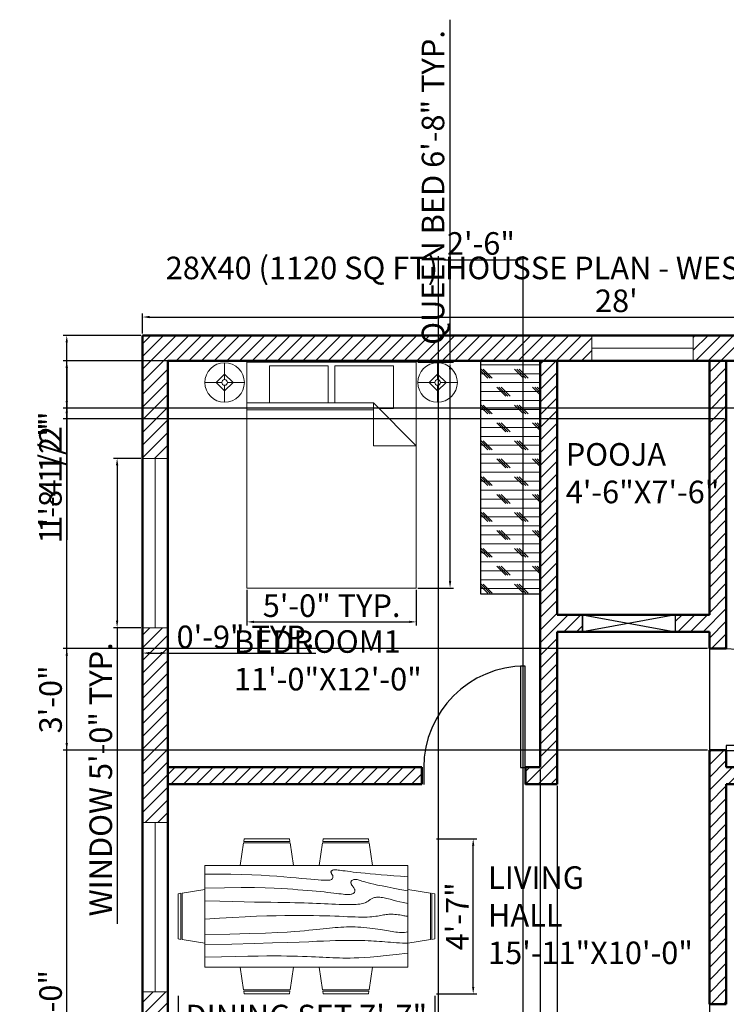
# Model space of a CAD drawing. Units: inches. Extents: x 1188 to 1681, y 1982 to 2608.
# Tile 3 of 4: x 1188 to 1439, y 2259 to 2608. Entities that reach past the tile are written whole.
import ezdxf

# ---------------------------------------------------------------- set-up
doc = ezdxf.new("R2010")
doc.units = ezdxf.units.IN
for name, color, linetype, lineweight in [('A-ANNO-DIMS', 2, 'Continuous', 18), ('A-ANNO-TEXT', 7, 'Continuous', 25), ('A-AREA-IDEN', 7, 'Continuous', 18), ('A-DOOR', 4, 'Continuous', 25), ('A-FLOR-CASE', 8, 'Continuous', 25), ('A-FLOR-CASE-PATT', 8, 'Continuous', 13), ('A-FURN', 8, 'Continuous', 18), ('A-GLAZ', 4, 'Continuous', 20), ('A-WALL', 7, 'Continuous', 50), ('A-WALL-PATT', 8, 'Continuous', 13)]:
    doc.layers.add(name, color=color, linetype=linetype, lineweight=lineweight)
doc.styles.get("Standard").update_dxf_attribs({"font": 'arial.ttf'})
doc.dimstyles.new('ISO-25', dxfattribs={"dimtxt": 8, "dimasz": 2.5, "dimexe": 1.25, "dimexo": 0.625, "dimtad": 1, "dimdec": 1, "dimlunit": 4, "dimtxsty": 'Standard', "dimcen": 2.5, "dimadec": 0, "dimazin": 0, "dimtfac": 1, "dimtdec": 1, "dimtmove": 0, "dimatfit": 3, "dimfxl": 1, "dimarcsym": 0})

# ---------------------------------------------------------------- blocks, each defined once
blk = doc.blocks.new('*U4')
for p, q in [((0, 0), (0, -6)), ((-36, 0), (-36, -6))]:
    blk.add_line(p, q)
blk.add_lwpolyline([(0, 0), (0, 36), (-1.75, 36), (-1.75, 0)], close=True)
blk.add_arc((0, 0), 36, 90, 180)
blk = doc.blocks.new('*U5')
for p, q in [((0, 0), (0, 6)), ((36, 0), (36, 6))]:
    blk.add_line(p, q)
blk.add_lwpolyline([(0, 0), (0, -36), (1.75, -36), (1.75, 0)], close=True)
blk.add_arc((0, 0), 36, 270, 0)
blk = doc.blocks.new('Bed - Queen')
for p, q in [((0, -80.00003), (0, 0)), ((0, 0), (59.99999, 0)), ((59.99999, 0), (59.99999, -80.00003)), ((7.99999, -1.2), (28.79998, -1.2)), ((7.99999, -14.4), (7.99999, -1.2)), ((28.79998, -1.2), (28.79998, -14.4)), ((31.19999, -1.2), (51.99999, -1.2)), ((31.19999, -14.4), (31.19999, -1.2)), ((51.99999, -1.2), (51.99999, -16.4)), ((0, -14.4), (44.8, -14.4)), ((44.8, -16.8), (0, -16.8)), ((59.99999, -29.6), (44.8, -14.4)), ((44.8, -14.4), (44.8, -29.6)), ((51.99999, -16.4), (46.79936, -16.4)), ((44.8, -29.6), (59.99999, -29.6)), ((59.99999, -80.00003), (0, -80.00003))]:
    blk.add_line(p, q)
blk = doc.blocks.new('Dining Set - 36 x 72 in.')
for p, q in [((-22.2343, 26.00059), (-23.4847, 17.99762)), ((-22.2304, 26), (-5.7608, 26)), ((-22, 27.5), (-22.1562, 26.50042)), ((-5.8416, 26.5), (-22.1534, 26.5)), ((-22, 27.5), (-6, 27.5)), ((-5.8437, 26.49966), (-6, 27.5)), ((-4.5152, 17.99762), (-5.7655, 25.99926)), ((5.7657, 26.00059), (4.5153, 17.99762)), ((5.7696, 26), (22.2392, 26)), ((6, 27.5), (5.8438, 26.50042)), ((22.1584, 26.5), (5.8466, 26.5)), ((6, 27.5), (22, 27.5)), ((22.1563, 26.49966), (22, 27.5)), ((23.4848, 17.99762), (22.2345, 25.99926)), ((36, 18), (-36, 18)), ((-36, 18), (-36, -18)), ((36, -18), (36, 18)), ((-45.5, 8), (-44.5004, 8.15617)), ((-45.5, 8), (-45.5, -8)), ((-44.5, -8.15843), (-44.5, 8.15338)), ((-44.0006, 8.23428), (-35.9976, 9.48474)), ((-44, 8.23041), (-44, -8.23915)), ((44.0006, 8.23428), (35.9976, 9.48474)), ((44, 8.23041), (44, -8.23915)), ((44.5, -8.15843), (44.5, 8.15338)), ((45.5, 8), (44.5005, 8.15617)), ((45.5, 8), (45.5, -8)), ((-44.4997, -8.15631), (-45.5, -8)), ((-35.9976, -9.48476), (-43.9993, -8.2345)), ((35.9976, -9.48476), (43.9993, -8.2345)), ((44.4997, -8.15631), (45.5, -8)), ((-36, -18), (36, -18)), ((-22.2343, -26.0006), (-23.4847, -17.99762)), ((-4.5152, -17.99762), (-5.7655, -25.99928)), ((5.7657, -26.0006), (4.5153, -17.99762)), ((23.4848, -17.99762), (22.2345, -25.99928)), ((-22.2304, -26), (-5.7608, -26)), ((-22, -27.5), (-22.1562, -26.50044)), ((-5.8416, -26.5), (-22.1534, -26.5)), ((-22, -27.5), (-6, -27.5)), ((-5.8437, -26.49967), (-6, -27.5)), ((5.7696, -26), (22.2392, -26)), ((6, -27.5), (5.8438, -26.50044)), ((22.1584, -26.5), (5.8466, -26.5)), ((6, -27.5), (22, -27.5)), ((22.1563, -26.49967), (22, -27.5))]:
    blk.add_line(p, q)
for points in [[(-36, 15), (-31.1772, 14.97754), (-26.8079, 14.91406), (-22.8538, 14.81543), (-19.276, 14.6875), (-16.0362, 14.53613), (-13.0957, 14.36718), (-10.4159, 14.18652), (-7.9583, 14), (-5.6904, 13.81315), (-3.6035, 13.63021), (-1.6954, 13.45508), (0.0365, 13.29166), (1.5945, 13.14388), (2.9811, 13.01562), (4.1988, 12.9108), (5.25, 12.83333), (6.1393, 12.78613), (6.8802, 12.76823), (7.4883, 12.77767), (7.9792, 12.8125), (8.3685, 12.87077), (8.6719, 12.95052), (8.9049, 13.0498), (9.0833, 13.16666), (9.2205, 13.29899), (9.3216, 13.44401), (9.3895, 13.59879), (9.4271, 13.76041), (9.4373, 13.92594), (9.4232, 14.09245), (9.3875, 14.257), (9.3333, 14.41666), (9.2638, 14.56917), (9.1836, 14.71484), (9.0975, 14.85465), (9.0104, 14.98958), (8.9272, 15.1206), (8.8529, 15.2487), (8.7922, 15.37483), (8.75, 15.5), (8.7305, 15.62467), (8.7344, 15.74739), (8.7617, 15.86621), (8.8125, 15.97916), (8.8867, 16.08431), (8.9844, 16.17968), (9.1055, 16.26334), (9.25, 16.33333), (9.4189, 16.38802), (9.6172, 16.42708), (9.8506, 16.45052), (10.125, 16.45833), (10.4463, 16.45052), (10.8203, 16.42708), (11.2529, 16.38802), (11.75, 16.33333), (12.3184, 16.26318), (12.9694, 16.17838), (13.7151, 16.07991), (14.5677, 15.96875), (15.5395, 15.84586), (16.6426, 15.71224), (17.8893, 15.56884), (19.2917, 15.41666), (20.859, 15.25667), (22.5879, 15.08984), (24.4721, 14.91715), (26.5052, 14.73958), (28.6809, 14.5581), (30.9929, 14.3737), (33.4347, 14.18733), (36, 14)], [(-36, 10), (-28.9766, 10.14274), (-23.1725, 10.20442), (-18.4241, 10.19775), (-14.5677, 10.13541), (-11.4399, 10.03011), (-8.877, 9.89453), (-6.7154, 9.74137), (-4.7917, 9.58333), (-2.9698, 9.43082), (-1.2246, 9.28515), (0.4415, 9.14534), (2.026, 9.01041), (3.5266, 8.87939), (4.9408, 8.7513), (6.266, 8.62516), (7.5, 8.5), (8.6411, 8.37549), (9.6914, 8.2539), (10.6538, 8.13818), (11.5312, 8.03125), (12.3267, 7.93603), (13.043, 7.85547), (13.6831, 7.79248), (14.25, 7.75), (14.7471, 7.7303), (15.1797, 7.73307), (15.5537, 7.75732), (15.875, 7.80208), (16.1494, 7.86637), (16.3828, 7.94922), (16.5811, 8.04964), (16.75, 8.16666), (16.8944, 8.29915), (17.0143, 8.44531), (17.1089, 8.60319), (17.1771, 8.77083), (17.218, 8.94629), (17.2305, 9.1276), (17.2137, 9.31282), (17.1667, 9.5), (17.0895, 9.6875), (16.987, 9.875), (16.8649, 10.0625), (16.7292, 10.25), (16.5856, 10.4375), (16.4401, 10.625), (16.2985, 10.8125), (16.1667, 11), (16.05, 11.18733), (15.9518, 11.3737), (15.8752, 11.5581), (15.8229, 11.73958), (15.798, 11.91715), (15.8034, 12.08984), (15.842, 12.25667), (15.9167, 12.41666), (16.0295, 12.56836), (16.1784, 12.70833), (16.3605, 12.83268), (16.5729, 12.9375), (16.8127, 13.01888), (17.0768, 13.07291), (17.3625, 13.0957), (17.6667, 13.08333), (17.9894, 13.03312), (18.3418, 12.94726), (18.7382, 12.82918), (19.1927, 12.68229), (19.7195, 12.51001), (20.3327, 12.31575), (21.0465, 12.10294), (21.875, 11.875), (22.8357, 11.63354), (23.959, 11.37304), (25.2786, 11.08618), (26.8282, 10.76562), (28.6414, 10.40405), (30.752, 9.99414), (33.1936, 9.52856), (36, 9)], [(-36, 5.5), (-30.7157, 5.3348), (-26.069, 5.20963), (-21.9946, 5.11767), (-18.4271, 5.05208), (-15.3009, 5.00602), (-12.5508, 4.97265), (-10.1112, 4.94515), (-7.9167, 4.91666), (-5.909, 4.88167), (-4.0586, 4.83984), (-2.3429, 4.79215), (-0.7396, 4.73958), (0.7739, 4.6831), (2.22, 4.6237), (3.6213, 4.56233), (5, 4.5), (6.373, 4.43782), (7.7344, 4.3776), (9.0723, 4.32129), (10.375, 4.27083), (11.6309, 4.22819), (12.8281, 4.19531), (13.9551, 4.17415), (15, 4.16666), (15.954, 4.17448), (16.819, 4.19791), (17.6001, 4.23698), (18.3021, 4.29166), (18.9299, 4.36198), (19.4883, 4.44791), (19.9823, 4.54948), (20.4167, 4.66666), (20.7969, 4.79899), (21.1302, 4.94401), (21.4245, 5.09879), (21.6875, 5.26041), (21.9271, 5.42594), (22.1511, 5.59245), (22.3672, 5.757), (22.5834, 5.91666), (22.8065, 6.06868), (23.0404, 6.21093), (23.2879, 6.34147), (23.5521, 6.45833), (23.8358, 6.55957), (24.142, 6.64323), (24.4735, 6.70735), (24.8334, 6.75), (25.2235, 6.76969), (25.642, 6.76692), (26.0858, 6.74267), (26.5521, 6.69791), (27.0379, 6.63362), (27.5404, 6.55078), (28.0565, 6.45036), (28.5834, 6.33333), (29.1242, 6.19987), (29.7071, 6.04687), (30.3661, 5.87044), (31.1354, 5.66666), (32.0493, 5.43164), (33.142, 5.16146), (34.4475, 4.85221), (36, 4.5)], [(-36, -1), (-30.7915, -0.6591), (-26.0195, -0.38216), (-21.6519, -0.16284), (-17.6563, 0.00521), (-14.0005, 0.12833), (-10.6523, 0.21289), (-7.5796, 0.26522), (-4.75, 0.29166), (-2.134, 0.29793), (0.2878, 0.28711), (2.5317, 0.26163), (4.6146, 0.22396), (6.5529, 0.17651), (8.3633, 0.12174), (10.0623, 0.06209), (11.6667, 0), (13.1899, -0.06201), (14.6341, -0.1211), (15.9982, -0.17432), (17.2813, -0.21875), (18.4823, -0.25147), (19.6003, -0.26953), (20.6343, -0.27002), (21.5834, -0.25), (22.4481, -0.20768), (23.2357, -0.14584), (23.9549, -0.06836), (24.6146, 0.02083), (25.2235, 0.11784), (25.7904, 0.21875), (26.3241, 0.31966), (26.8334, 0.41666), (27.3265, 0.50618), (27.8099, 0.58593), (28.2894, 0.65397), (28.7709, 0.70833), (29.2601, 0.74707), (29.763, 0.76823), (30.2855, 0.76985), (30.8334, 0.75), (31.4088, 0.70784), (31.9994, 0.64713), (32.589, 0.57275), (33.1615, 0.48958), (33.7008, 0.4025), (34.1908, 0.3164), (34.6153, 0.23616), (34.9584, 0.16666), (35.2099, 0.11165), (35.3848, 0.07031), (35.504, 0.04069), (35.5886, 0.02083), (35.6594, 0.00879), (35.7377, 0.0026), (35.8442, 0.00032), (36, 0)], [(-36, -6.5), (-27.1843, -6.31267), (-20.084, -6.1263), (-14.469, -5.9419), (-10.1094, -5.76042), (-6.7752, -5.58285), (-4.2363, -5.41016), (-2.2629, -5.24333), (-0.625, -5.08334), (0.8708, -4.93099), (2.2715, -4.78646), (3.5872, -4.64974), (4.8281, -4.52084), (6.0046, -4.39974), (7.127, -4.28646), (8.2053, -4.18099), (9.25, -4.08334), (10.2705, -3.99382), (11.2734, -3.91407), (12.2647, -3.84603), (13.25, -3.79167), (14.2354, -3.75293), (15.2266, -3.73177), (16.2295, -3.73015), (17.25, -3.75), (18.2912, -3.79248), (19.3451, -3.85547), (20.4009, -3.93604), (21.4479, -4.03125), (22.4754, -4.13819), (23.4727, -4.25391), (24.4289, -4.37549), (25.3334, -4.5), (26.1785, -4.62492), (26.9694, -4.74935), (27.7145, -4.87281), (28.4219, -4.99479), (29.1, -5.11483), (29.7572, -5.23242), (30.4016, -5.34709), (31.0417, -5.45834), (31.6837, -5.56437), (32.3262, -5.65821), (32.9658, -5.73153), (33.599, -5.77604), (34.2224, -5.78345), (34.8327, -5.74545), (35.4264, -5.65373), (36, -5.5)], [(-36, -10), (-26.4022, -9.81299), (-18.4675, -9.62891), (-11.9839, -9.45069), (-6.7396, -9.28125), (-2.5226, -9.12354), (0.8789, -8.98047), (3.6769, -8.85498), (6.0833, -8.75), (8.2767, -8.66765), (10.3021, -8.60677), (12.1712, -8.56543), (13.8958, -8.54167), (15.4876, -8.53353), (16.9583, -8.53907), (18.3197, -8.55632), (19.5834, -8.58334), (20.7616, -8.61841), (21.8685, -8.66081), (22.9188, -8.71004), (23.9271, -8.76563), (24.9081, -8.82707), (25.8763, -8.89388), (26.8465, -8.96558), (27.8334, -9.04167), (28.8474, -9.12118), (29.8828, -9.20117), (30.93, -9.27824), (31.9792, -9.34896), (33.0205, -9.40991), (34.0443, -9.45768), (35.0407, -9.48885), (36, -9.5)], [(-36, -14.5), (-30.0881, -14.33513), (-25.0332, -14.21224), (-20.7312, -14.12647), (-17.0781, -14.07292), (-13.97, -14.04671), (-11.3027, -14.04297), (-8.9724, -14.05681), (-6.875, -14.08334), (-4.9224, -14.11833), (-3.0905, -14.16016), (-1.3709, -14.20785), (0.2448, -14.26042), (1.7647, -14.3169), (3.1973, -14.3763), (4.5507, -14.43767), (5.8333, -14.5), (7.0554, -14.5621), (8.235, -14.62175), (9.3922, -14.67652), (10.5469, -14.72396), (11.7192, -14.76164), (12.929, -14.78711), (14.1965, -14.79794), (15.5417, -14.79167), (16.9933, -14.76424), (18.6152, -14.70508), (20.4804, -14.60197), (22.6615, -14.44271), (25.2312, -14.21509), (28.2624, -13.9069), (31.8277, -13.50594), (36, -13)]]:
    blk.add_lwpolyline(points)
blk = doc.blocks.new('Lamp - Table')
for p, q in [((0, 7), (0, 1)), ((-1, 0), (-7, 0)), ((0, 3), (-3, 0)), ((-3, 0), (0, -3)), ((3, 0), (0, 3)), ((0, -3), (3, 0)), ((1, 0), (7, 0)), ((0, -1), (0, -7))]:
    blk.add_line(p, q)
for radius in [7, 1]:
    blk.add_circle((0, 0), radius)
blk = doc.blocks.new('*D14')
at = {"layer": 'A-ANNO-DIMS', "color": 0, "lineweight": -2, "transparency": 16777216}
for p, q in [((1231.72, 2497.04), (1231.72, 2504.18)), ((1234.22, 2502.93), (1565.22, 2502.93)), ((1567.72, 2497.04), (1567.72, 2504.18))]:
    blk.add_line(p, q, dxfattribs=at)
at = {"layer": 'A-ANNO-DIMS', "color": 0, "transparency": 16777216}
for points in [[(1234.22, 2503.35), (1234.22, 2502.52), (1231.72, 2502.93)], [(1565.22, 2503.35), (1565.22, 2502.52), (1567.72, 2502.93)]]:
    blk.add_solid(points, dxfattribs=at)
at = {"layer": 'Defpoints', "color": 0, "transparency": 16777216}
for p in [(1567.72, 2502.93), (1231.72, 2496.41), (1567.72, 2496.41)]:
    blk.add_point(p, dxfattribs=at)
at = {"layer": 'A-ANNO-DIMS', "color": 0, "transparency": 16777216, "insert": (1399.72, 2507.64), "char_height": 8, "attachment_point": 5}
blk.add_mtext("28'", dxfattribs=at)
blk = doc.blocks.new('WIN-60IN')
for p, q in [((0, 9), (0, 0)), ((60, 0), (60, 9)), ((60, 9), (60, 4.5)), ((60, 4.5), (0, 4.5)), ((0, 0), (60, 0))]:
    blk.add_line(p, q)
blk = doc.blocks.new('*D24')
at = {"layer": 'A-ANNO-DIMS', "color": 0, "lineweight": -2, "transparency": 16777216}
for p, q in [((1231.09, 2452.82), (1221.47, 2452.82)), ((1222.72, 2450.32), (1222.72, 2395.32)), ((1231.09, 2392.82), (1221.47, 2392.82)), ((1222.72, 2392.82), (1222.72, 2287.84))]:
    blk.add_line(p, q, dxfattribs=at)
at = {"layer": 'A-ANNO-DIMS', "color": 0, "transparency": 16777216}
for points in [[(1222.3, 2450.32), (1223.13, 2450.32), (1222.72, 2452.82)], [(1222.3, 2395.32), (1223.13, 2395.32), (1222.72, 2392.82)]]:
    blk.add_solid(points, dxfattribs=at)
at = {"layer": 'Defpoints', "color": 0, "transparency": 16777216}
for p in [(1231.72, 2452.82), (1222.72, 2392.82), (1231.72, 2392.82)]:
    blk.add_point(p, dxfattribs=at)
at = {"layer": 'A-ANNO-DIMS', "color": 0, "transparency": 16777216, "insert": (1217.95, 2339.08), "char_height": 8, "attachment_point": 5, "rotation": 90}
blk.add_mtext('WINDOW 5\'-0" TYP.', dxfattribs=at)
blk = doc.blocks.new('*D25')
at = {"layer": 'A-ANNO-DIMS', "color": 0, "lineweight": -2, "transparency": 16777216}
for p, q in [((1231.72, 2392.2), (1231.72, 2382.57)), ((1240.72, 2392.2), (1240.72, 2382.57)), ((1234.22, 2383.82), (1238.22, 2383.82)), ((1240.72, 2383.82), (1293.23, 2383.82))]:
    blk.add_line(p, q, dxfattribs=at)
at = {"layer": 'A-ANNO-DIMS', "color": 0, "transparency": 16777216}
for points in [[(1234.22, 2384.24), (1234.22, 2383.41), (1231.72, 2383.82)], [(1238.22, 2384.24), (1238.22, 2383.41), (1240.72, 2383.82)]]:
    blk.add_solid(points, dxfattribs=at)
at = {"layer": 'Defpoints', "color": 0, "transparency": 16777216}
for p in [(1231.72, 2392.82), (1240.72, 2392.82), (1240.72, 2383.82)]:
    blk.add_point(p, dxfattribs=at)
at = {"layer": 'A-ANNO-DIMS', "color": 0, "transparency": 16777216, "insert": (1268.22, 2388.53), "char_height": 8, "attachment_point": 5}
blk.add_mtext('0\'-9" TYP.', dxfattribs=at)
blk = doc.blocks.new('*D28')
at = {"layer": 'A-ANNO-DIMS', "color": 0, "lineweight": -2, "transparency": 16777216}
for p, q in [((1340.77, 2486.88), (1340.77, 2608.31)), ((1329.39, 2486.88), (1342.02, 2486.88)), ((1340.77, 2409.38), (1340.77, 2484.38)), ((1329.39, 2406.88), (1342.02, 2406.88))]:
    blk.add_line(p, q, dxfattribs=at)
at = {"layer": 'A-ANNO-DIMS', "color": 0, "transparency": 16777216}
for points in [[(1340.35, 2484.38), (1341.18, 2484.38), (1340.77, 2486.88)], [(1340.35, 2409.38), (1341.18, 2409.38), (1340.77, 2406.88)]]:
    blk.add_solid(points, dxfattribs=at)
at = {"layer": 'Defpoints', "color": 0, "transparency": 16777216}
for p in [(1328.77, 2486.88), (1340.77, 2486.88), (1328.77, 2406.88)]:
    blk.add_point(p, dxfattribs=at)
at = {"layer": 'A-ANNO-DIMS', "color": 0, "transparency": 16777216, "insert": (1335.76, 2548.85), "char_height": 8, "attachment_point": 5, "rotation": 90}
blk.add_mtext('QUEEN BED 6\'-8" TYP.', dxfattribs=at)
blk = doc.blocks.new('*D29')
at = {"layer": 'A-ANNO-DIMS', "color": 0, "lineweight": -2, "transparency": 16777216}
for p, q in [((1268.77, 2406.26), (1268.77, 2393.63)), ((1328.77, 2406.26), (1328.77, 2393.63)), ((1271.27, 2394.88), (1326.27, 2394.88))]:
    blk.add_line(p, q, dxfattribs=at)
at = {"layer": 'A-ANNO-DIMS', "color": 0, "transparency": 16777216}
for points in [[(1271.27, 2395.3), (1271.27, 2394.47), (1268.77, 2394.88)], [(1326.27, 2395.3), (1326.27, 2394.47), (1328.77, 2394.88)]]:
    blk.add_solid(points, dxfattribs=at)
at = {"layer": 'Defpoints', "color": 0, "transparency": 16777216}
for p in [(1268.77, 2406.88), (1328.77, 2406.88), (1328.77, 2394.88)]:
    blk.add_point(p, dxfattribs=at)
at = {"layer": 'A-ANNO-DIMS', "color": 0, "transparency": 16777216, "insert": (1298.77, 2399.59), "char_height": 8, "attachment_point": 5}
blk.add_mtext('5\'-0" TYP.', dxfattribs=at)
blk = doc.blocks.new('*D38')
at = {"layer": 'A-ANNO-DIMS', "color": 0, "lineweight": -2, "transparency": 16777216}
for p, q in [((1244.32, 2262.4), (1244.32, 2248.12)), ((1335.32, 2262.4), (1335.32, 2248.12)), ((1246.82, 2249.37), (1332.82, 2249.37))]:
    blk.add_line(p, q, dxfattribs=at)
at = {"layer": 'A-ANNO-DIMS', "color": 0, "transparency": 16777216}
for points in [[(1246.82, 2249.79), (1246.82, 2248.96), (1244.32, 2249.37)], [(1332.82, 2249.79), (1332.82, 2248.96), (1335.32, 2249.37)]]:
    blk.add_solid(points, dxfattribs=at)
at = {"layer": 'Defpoints', "color": 0, "transparency": 16777216}
for p in [(1244.32, 2263.02), (1335.32, 2263.02), (1335.32, 2249.37)]:
    blk.add_point(p, dxfattribs=at)
at = {"layer": 'A-ANNO-DIMS', "color": 0, "transparency": 16777216, "insert": (1289.82, 2254.14), "char_height": 8, "attachment_point": 5}
blk.add_mtext('DINING SET 7\'-7"', dxfattribs=at)
blk = doc.blocks.new('*D39')
at = {"layer": 'A-ANNO-DIMS', "color": 0, "lineweight": -2, "transparency": 16777216}
for p, q in [((1335.95, 2318.02), (1350.22, 2318.02)), ((1348.97, 2265.52), (1348.97, 2315.52)), ((1335.95, 2263.02), (1350.22, 2263.02))]:
    blk.add_line(p, q, dxfattribs=at)
at = {"layer": 'A-ANNO-DIMS', "color": 0, "transparency": 16777216}
for points in [[(1348.56, 2315.52), (1349.39, 2315.52), (1348.97, 2318.02)], [(1348.56, 2265.52), (1349.39, 2265.52), (1348.97, 2263.02)]]:
    blk.add_solid(points, dxfattribs=at)
at = {"layer": 'Defpoints', "color": 0, "transparency": 16777216}
for p in [(1335.32, 2318.02), (1348.97, 2318.02), (1335.32, 2263.02)]:
    blk.add_point(p, dxfattribs=at)
at = {"layer": 'A-ANNO-DIMS', "color": 0, "transparency": 16777216, "insert": (1344.35, 2290.52), "char_height": 8, "attachment_point": 5, "rotation": 90}
blk.add_mtext('4\'-7"', dxfattribs=at)
blk = doc.blocks.new('*D44')
at = {"layer": 'A-ANNO-DIMS', "color": 0, "lineweight": -2, "transparency": 16777216}
for p, q in [((1231.09, 2496.41), (1203.62, 2496.41)), ((1204.87, 2018.91), (1204.87, 2493.91)), ((1231.09, 2016.41), (1203.62, 2016.41))]:
    blk.add_line(p, q, dxfattribs=at)
at = {"layer": 'A-ANNO-DIMS', "color": 0, "transparency": 16777216}
for points in [[(1204.45, 2493.91), (1205.28, 2493.91), (1204.87, 2496.41)], [(1204.45, 2018.91), (1205.28, 2018.91), (1204.87, 2016.41)]]:
    blk.add_solid(points, dxfattribs=at)
at = {"layer": 'Defpoints', "color": 0, "transparency": 16777216}
for p in [(1204.87, 2496.41), (1231.72, 2496.41), (1231.72, 2016.41)]:
    blk.add_point(p, dxfattribs=at)
at = {"layer": 'A-ANNO-DIMS', "color": 0, "transparency": 16777216, "insert": (1200.16, 2256.41), "char_height": 8, "attachment_point": 5, "rotation": 90}
blk.add_mtext('40\'-0"', dxfattribs=at)
blk = doc.blocks.new('*D47')
at = {"layer": 'A-ANNO-DIMS', "color": 0, "lineweight": -2, "transparency": 16777216}
for p, q in [((1336.72, 2164.04), (1336.72, 2524.51)), ((1339.22, 2523.26), (1364.22, 2523.26)), ((1366.72, 2164.04), (1366.72, 2524.51))]:
    blk.add_line(p, q, dxfattribs=at)
at = {"layer": 'A-ANNO-DIMS', "color": 0, "transparency": 16777216}
for points in [[(1339.22, 2523.68), (1339.22, 2522.85), (1336.72, 2523.26)], [(1364.22, 2523.68), (1364.22, 2522.85), (1366.72, 2523.26)]]:
    blk.add_solid(points, dxfattribs=at)
at = {"layer": 'Defpoints', "color": 0, "transparency": 16777216}
for p in [(1366.72, 2523.26), (1336.72, 2163.41), (1366.72, 2163.41)]:
    blk.add_point(p, dxfattribs=at)
at = {"layer": 'A-ANNO-DIMS', "color": 0, "transparency": 16777216, "insert": (1351.72, 2527.97), "char_height": 8, "attachment_point": 5}
blk.add_mtext('2\'-6"', dxfattribs=at)
blk = doc.blocks.new('*D50')
at = {"layer": 'A-ANNO-DIMS', "color": 0, "lineweight": -2, "transparency": 16777216}
for p, q in [((1372.72, 2342.79), (1372.72, 1988.31)), ((1378.72, 2336.79), (1378.72, 1988.31)), ((1370.22, 1989.56), (1367.72, 1989.56)), ((1372.72, 1989.56), (1378.72, 1989.56)), ((1381.22, 1989.56), (1406.23, 1989.56))]:
    blk.add_line(p, q, dxfattribs=at)
at = {"layer": 'A-ANNO-DIMS', "color": 0, "transparency": 16777216}
for points in [[(1370.22, 1989.98), (1370.22, 1989.15), (1372.72, 1989.56)], [(1381.22, 1989.98), (1381.22, 1989.15), (1378.72, 1989.56)]]:
    blk.add_solid(points, dxfattribs=at)
at = {"layer": 'Defpoints', "color": 0, "transparency": 16777216}
for p in [(1372.72, 2343.41), (1378.72, 2337.41), (1378.72, 1989.56)]:
    blk.add_point(p, dxfattribs=at)
at = {"layer": 'A-ANNO-DIMS', "color": 0, "transparency": 16777216, "insert": (1394.97, 1994.27), "char_height": 8, "attachment_point": 5}
blk.add_mtext('0\'-6"', dxfattribs=at)
blk = doc.blocks.new('*D51')
at = {"layer": 'A-ANNO-DIMS', "color": 0, "lineweight": -2, "transparency": 16777216}
for p, q in [((1438.09, 2487.41), (1203.62, 2487.41)), ((1204.87, 2484.91), (1204.87, 2469.37)), ((1438.09, 2466.87), (1203.62, 2466.87)), ((1204.87, 2466.87), (1204.87, 2423.97))]:
    blk.add_line(p, q, dxfattribs=at)
at = {"layer": 'A-ANNO-DIMS', "color": 0, "transparency": 16777216}
for points in [[(1204.45, 2484.91), (1205.28, 2484.91), (1204.87, 2487.41)], [(1204.45, 2469.37), (1205.28, 2469.37), (1204.87, 2466.87)]]:
    blk.add_solid(points, dxfattribs=at)
at = {"layer": 'Defpoints', "color": 0, "transparency": 16777216}
for p in [(1438.72, 2487.41), (1204.87, 2466.87), (1438.72, 2466.87)]:
    blk.add_point(p, dxfattribs=at)
at = {"layer": 'A-ANNO-DIMS', "color": 0, "transparency": 16777216, "insert": (1200.11, 2444.17), "char_height": 8, "attachment_point": 5, "rotation": 90}
blk.add_mtext('1\'-8 1/2"', dxfattribs=at)
blk = doc.blocks.new('*D54')
at = {"layer": 'A-ANNO-DIMS', "color": 0, "lineweight": -2, "transparency": 16777216}
for p, q in [((1479.32, 2487.41), (1203.62, 2487.41)), ((1204.87, 2484.91), (1204.87, 2473.18)), ((1479.32, 2470.68), (1203.62, 2470.68)), ((1204.87, 2470.68), (1204.87, 2427.77))]:
    blk.add_line(p, q, dxfattribs=at)
at = {"layer": 'A-ANNO-DIMS', "color": 0, "transparency": 16777216}
for points in [[(1204.45, 2484.91), (1205.28, 2484.91), (1204.87, 2487.41)], [(1204.45, 2473.18), (1205.28, 2473.18), (1204.87, 2470.68)]]:
    blk.add_solid(points, dxfattribs=at)
at = {"layer": 'Defpoints', "color": 0, "transparency": 16777216}
for p in [(1479.94, 2487.41), (1204.87, 2470.68), (1479.94, 2470.68)]:
    blk.add_point(p, dxfattribs=at)
at = {"layer": 'A-ANNO-DIMS', "color": 0, "transparency": 16777216, "insert": (1200.11, 2447.98), "char_height": 8, "attachment_point": 5, "rotation": 90}
blk.add_mtext('1\'-4 1/2"', dxfattribs=at)
blk = doc.blocks.new('*D55')
at = {"layer": 'A-ANNO-DIMS', "color": 0, "lineweight": -2, "transparency": 16777216}
for p, q in [((1432.09, 2385.41), (1203.62, 2385.41)), ((1204.87, 2351.91), (1204.87, 2382.91)), ((1432.09, 2349.41), (1203.62, 2349.41))]:
    blk.add_line(p, q, dxfattribs=at)
at = {"layer": 'A-ANNO-DIMS', "color": 0, "transparency": 16777216}
for points in [[(1204.45, 2382.91), (1205.28, 2382.91), (1204.87, 2385.41)], [(1204.45, 2351.91), (1205.28, 2351.91), (1204.87, 2349.41)]]:
    blk.add_solid(points, dxfattribs=at)
at = {"layer": 'Defpoints', "color": 0, "transparency": 16777216}
for p in [(1204.87, 2385.41), (1432.72, 2385.41), (1432.72, 2349.41)]:
    blk.add_point(p, dxfattribs=at)
at = {"layer": 'A-ANNO-DIMS', "color": 0, "transparency": 16777216, "insert": (1200.15, 2367.41), "char_height": 8, "attachment_point": 5, "rotation": 90}
blk.add_mtext('3\'-0"', dxfattribs=at)

msp = doc.modelspace()

# ---------------------------------------------------------------- hatches: boundary and pattern name
at = {"layer": 'A-FLOR-CASE-PATT', "transparency": 33554564}
h = msp.add_hatch(dxfattribs=at)
h.set_pattern_fill('CORK', color=256)
h.set_pattern_definition([(0, (0, 0), (0, 3.175), []), (135, (1.5875, -1.5875), (-6.350003, -6.350003), [4.49013, -4.49013]), (135, (2.381, -1.5875), (-6.350003, -6.350003), [4.49013, -4.49013]), (135, (3.175, -1.5875), (-6.350003, -6.350003), [4.49013, -4.49013])])
h.paths.add_polyline_path([(1372.72, 2487.41), (1351.56, 2487.41), (1351.56, 2404.84), (1372.72, 2404.84)])
at = {"layer": 'A-WALL-PATT', "transparency": 33554559}
h = msp.add_hatch(dxfattribs=at)
h.set_pattern_fill('ANSI31', color=256)
h.paths.add_polyline_path([(1390.99, 2496.41), (1231.72, 2496.41), (1231.72, 2452.82), (1240.72, 2452.82), (1240.72, 2487.41), (1390.99, 2487.41)])
h.paths.add_polyline_path([(1469.3, 2496.41), (1426.99, 2496.41), (1426.99, 2491.91), (1426.99, 2487.41), (1469.3, 2487.41)])
h.paths.add_polyline_path([(1378.72, 2487.41), (1372.72, 2487.41), (1372.72, 2404.84), (1372.72, 2343.41), (1367.48, 2343.41), (1367.48, 2337.41), (1378.72, 2337.41), (1378.72, 2391.41), (1387.67, 2391.41), (1387.67, 2397.41), (1378.72, 2397.41)])
h.paths.add_polyline_path([(1438.72, 2487.41), (1432.72, 2487.41), (1432.72, 2397.41), (1420.72, 2397.41), (1420.72, 2391.41), (1432.72, 2391.41), (1432.72, 2385.41), (1438.72, 2385.41)])
h.paths.add_polyline_path([(1240.72, 2392.82), (1236.22, 2392.82), (1231.72, 2392.82), (1231.72, 2323.77), (1240.72, 2323.77)])
h.paths.add_polyline_path([(1330.72, 2343.41), (1240.72, 2343.41), (1240.72, 2337.41), (1330.72, 2337.41)])
h.paths.add_polyline_path([(1558.72, 2343.41), (1438.72, 2343.41), (1438.72, 2349.29), (1438.64, 2349.29), (1432.72, 2349.29), (1432.72, 2259.41), (1438.72, 2259.41), (1438.72, 2337.41), (1558.72, 2337.41)])
h.paths.add_polyline_path([(1567.72, 2396.81), (1558.72, 2396.81), (1558.72, 2317.68), (1563.22, 2317.68), (1567.72, 2317.68)])
h.paths.add_polyline_path([(1567.72, 2496.41), (1529.3, 2496.41), (1529.3, 2491.91), (1529.3, 2487.41), (1558.72, 2487.41), (1558.72, 2461.81), (1567.72, 2461.81)])
h.paths.add_polyline_path([(1240.72, 2195.41), (1240.72, 2201.41), (1240.72, 2263.77), (1231.72, 2263.77), (1231.72, 2016.41), (1246.72, 2016.41), (1246.72, 2022.41), (1246.72, 2025.41), (1240.72, 2025.41)])
h.paths.add_polyline_path([(1391.72, 2211.41), (1397.72, 2211.41), (1397.72, 2217.41), (1385.72, 2217.41), (1385.72, 2163.41), (1366.72, 2163.41), (1366.72, 2157.41), (1385.72, 2157.41), (1385.72, 2073.41), (1391.72, 2073.41)])
h.paths.add_polyline_path([(1330.72, 2201.41), (1282.72, 2201.41), (1282.72, 2195.41), (1324.72, 2195.41), (1324.72, 2064.41), (1345.75, 2064.41), (1345.75, 2073.41), (1330.72, 2073.41), (1330.72, 2157.41), (1336.72, 2157.41), (1336.72, 2163.41), (1330.72, 2163.41)])
h.paths.add_polyline_path([(1558.72, 2217.41), (1438.72, 2217.41), (1438.72, 2223.26), (1432.72, 2223.26), (1432.72, 2217.41), (1427.72, 2217.41), (1427.72, 2211.41), (1432.72, 2211.41), (1558.72, 2211.41)])
h.paths.add_polyline_path([(1567.72, 2269.68), (1558.72, 2269.68), (1558.72, 2182.72), (1563.22, 2182.72), (1567.72, 2182.72)])
h.paths.add_polyline_path([(1567.72, 2134.72), (1558.72, 2134.72), (1558.72, 2073.41), (1497.85, 2073.41), (1497.85, 2068.91), (1497.85, 2064.41), (1567.72, 2064.41)])
h.paths.add_polyline_path([(1449.85, 2073.41), (1371.31, 2073.41), (1371.31, 2068.91), (1371.31, 2064.41), (1449.85, 2064.41)])
h.paths.add_polyline_path([(1333.72, 2064.41), (1324.72, 2064.41), (1324.72, 2025.41), (1313.9, 2025.41), (1313.9, 2016.41), (1333.72, 2016.41)])

# ---------------------------------------------------------------- linework, layer by layer
at = {"layer": 'A-DOOR'}
for p, q in [((1387.67, 2397.41), (1387.67, 2391.41)), ((1420.72, 2397.41), (1387.67, 2391.41)), ((1387.67, 2391.41), (1387.67, 2397.41)), ((1387.67, 2397.41), (1420.72, 2391.41)), ((1420.72, 2391.41), (1420.72, 2397.41)), ((1387.67, 2391.41), (1420.72, 2391.41)), ((1432.72, 2385.41), (1432.72, 2349.41)), ((1432.72, 2259.41), (1432.72, 2223.41))]:
    msp.add_line(p, q, dxfattribs=at)
at = {"layer": 'A-FLOR-CASE'}
msp.add_lwpolyline([(1372.72, 2487.41), (1351.56, 2487.41), (1351.56, 2404.84), (1372.72, 2404.84)], close=True, dxfattribs=at)
at = {"layer": 'A-GLAZ'}
for p, q in [((1390.99, 2496.41), (1390.99, 2487.41)), ((1426.99, 2487.41), (1426.99, 2496.41)), ((1426.99, 2496.41), (1426.99, 2491.91)), ((1426.99, 2491.91), (1390.99, 2491.91)), ((1390.99, 2487.41), (1426.99, 2487.41))]:
    msp.add_line(p, q, dxfattribs=at)
at = {"layer": 'A-WALL'}
for p, q in [((1231.72, 2496.41), (1231.72, 2016.41)), ((1231.72, 2496.41), (1567.72, 2496.41)), ((1240.72, 2487.41), (1558.72, 2487.41)), ((1240.72, 2487.41), (1240.72, 2201.41)), ((1372.72, 2487.41), (1372.72, 2343.41)), ((1378.72, 2487.41), (1378.72, 2397.41)), ((1432.72, 2487.41), (1432.72, 2397.41)), ((1438.72, 2487.41), (1438.72, 2385.41)), ((1378.72, 2397.41), (1432.72, 2397.41)), ((1378.72, 2391.41), (1432.72, 2391.41)), ((1378.72, 2391.41), (1378.72, 2337.41)), ((1432.72, 2391.41), (1432.72, 2385.41)), ((1432.72, 2385.41), (1438.72, 2385.41)), ((1432.72, 2349.41), (1438.72, 2349.41)), ((1432.72, 2349.41), (1432.72, 2259.41)), ((1438.72, 2349.41), (1438.72, 2343.41)), ((1240.72, 2343.41), (1330.72, 2343.41)), ((1330.72, 2343.41), (1330.72, 2337.41)), ((1367.48, 2343.41), (1372.72, 2343.41)), ((1367.48, 2343.41), (1367.48, 2337.41)), ((1438.72, 2343.41), (1558.72, 2343.41)), ((1330.72, 2337.41), (1240.72, 2337.41)), ((1367.48, 2337.41), (1378.72, 2337.41)), ((1438.72, 2337.41), (1558.72, 2337.41)), ((1438.72, 2337.41), (1438.72, 2259.41)), ((1432.72, 2259.41), (1438.72, 2259.41))]:
    msp.add_line(p, q, dxfattribs=at)

# ---------------------------------------------------------------- block references
at = {"layer": 'A-DOOR', "rotation": 90}
msp.add_blockref('*U5', (1438.64, 2349.29), dxfattribs=at)
at = {"layer": 'A-DOOR'}
msp.add_blockref('*U4', (1367.44, 2343.23), dxfattribs=at)
at = {"layer": 'A-FURN'}
for name, p in [('Lamp - Table', (1260.84, 2479.73)), ('Bed - Queen', (1268.77, 2486.88)), ('Lamp - Table', (1336.36, 2479.73)), ('Dining Set - 36 x 72 in.', (1289.82, 2290.52))]:
    msp.add_blockref(name, p, dxfattribs=at)
at = {"layer": 'A-GLAZ', "rotation": 270.0000000000002}
msp.add_blockref('WIN-60IN', (1231.72, 2452.82), dxfattribs=at)
at = {"layer": 'A-GLAZ', "extrusion": (0, 0, -1), "zscale": -1, "rotation": 269.9999999999992}
msp.add_blockref('WIN-60IN', (-1240.72, 2323.77), dxfattribs=at)

# ---------------------------------------------------------------- texts
at = {"layer": 'A-ANNO-TEXT', "insert": (1239.94, 2524.33), "char_height": 8, "attachment_point": 1}
msp.add_mtext('28X40 (1120 SQ FT) HOUSSE PLAN - WEST FACE -FP1316', dxfattribs=at)
at = {"layer": 'A-AREA-IDEN', "insert": (1381.79, 2458.25), "char_height": 8, "attachment_point": 1}
msp.add_mtext('POOJA \\P4\'-6"X7\'-6"', dxfattribs=at)
at = {"layer": 'A-AREA-IDEN', "char_height": 8, "attachment_point": 1}
for s, width, insert in [('BEDROOM1\\P11\'-0"X12\'-0"', 2.2674, (1264.15, 2391.92)), ('LIVING HALL\\P15\'-11"X10\'-0"', 0.7677, (1354.23, 2308.25))]:
    msp.add_mtext_dynamic_manual_height_columns(s, width=width, gutter_width=12.5, heights=[0], dxfattribs=dict(at, insert=insert))

# ---------------------------------------------------------------- dimensions: what is measured, and where the dimension line sits
at = {"layer": 'A-ANNO-DIMS'}
for base, p1, p2, angle, text, picture, middle in [((1340.77, 2486.88), (1328.77, 2406.88), (1328.77, 2486.88), 90, 'QUEEN BED <> TYP.', '*D28', (1335.76, 2548.85)), ((1222.72, 2392.82), (1231.72, 2452.82), (1231.72, 2392.82), 270, 'WINDOW <> TYP.', '*D24', (1217.95, 2339.08))]:
    dim = msp.add_linear_dim(base=base, p1=p1, p2=p2, angle=angle, text=text, dimstyle='ISO-25', override={"dimdec": 1, "dimlfac": 1, "dimrnd": 0, "dimzin": 1, "dimdsep": 46, "dimlunit": 4, "dimfrac": 2}, dxfattribs=at)
    dim.commit()
    dim.dimension.update_dxf_attribs({"geometry": picture, "text_midpoint": middle})
for base, p1, p2, override, picture, middle in [((1366.72, 2523.26), (1336.72, 2163.41), (1366.72, 2163.41), {"dimdec": 1, "dimlfac": 1, "dimrnd": 0, "dimzin": 1, "dimdsep": 46, "dimlunit": 4, "dimfrac": 2}, '*D47', (1351.72, 2527.97)), ((1567.72, 2502.93), (1231.72, 2496.41), (1567.72, 2496.41), {"dimclrd": 0, "dimclre": 0, "dimclrt": 0}, '*D14', (1399.72, 2507.64)), ((1378.72, 1989.56), (1372.72, 2343.41), (1378.72, 2337.41), {"dimdec": 1, "dimlfac": 1, "dimrnd": 0, "dimzin": 1, "dimdsep": 46, "dimlunit": 4, "dimfrac": 2}, '*D50', (1394.97, 1994.27))]:
    dim = msp.add_linear_dim(base=base, p1=p1, p2=p2, dimstyle='ISO-25', override=override, dxfattribs=at)
    dim.commit()
    dim.dimension.update_dxf_attribs({"geometry": picture, "text_midpoint": middle})
for base, p1, p2, picture, middle in [((1204.87, 2496.41), (1231.72, 2016.41), (1231.72, 2496.41), '*D44', (1200.16, 2256.41)), ((1204.87, 2466.87), (1438.72, 2487.41), (1438.72, 2466.87), '*D51', (1200.11, 2444.17)), ((1204.87, 2470.68), (1479.94, 2487.41), (1479.94, 2470.68), '*D54', (1200.11, 2447.98)), ((1204.87, 2385.41), (1432.72, 2349.41), (1432.72, 2385.41), '*D55', (1200.15, 2367.41)), ((1348.97, 2318.02), (1335.32, 2263.02), (1335.32, 2318.02), '*D39', (1344.35, 2290.52))]:
    dim = msp.add_linear_dim(base=base, p1=p1, p2=p2, angle=90, dimstyle='ISO-25', override={"dimdec": 1, "dimlfac": 1, "dimrnd": 0, "dimzin": 1, "dimdsep": 46, "dimlunit": 4, "dimfrac": 2}, dxfattribs=at)
    dim.commit()
    dim.dimension.update_dxf_attribs({"geometry": picture, "text_midpoint": middle})
for base, p1, p2, text, picture, middle in [((1328.77, 2394.88), (1268.77, 2406.88), (1328.77, 2406.88), '<> TYP.', '*D29', (1298.77, 2399.59)), ((1240.72, 2383.82), (1231.72, 2392.82), (1240.72, 2392.82), '<> TYP.', '*D25', (1268.22, 2388.53)), ((1335.32, 2249.37), (1244.32, 2263.02), (1335.32, 2263.02), 'DINING SET <>', '*D38', (1289.82, 2254.14))]:
    dim = msp.add_linear_dim(base=base, p1=p1, p2=p2, text=text, dimstyle='ISO-25', override={"dimdec": 1, "dimlfac": 1, "dimrnd": 0, "dimzin": 1, "dimdsep": 46, "dimlunit": 4, "dimfrac": 2}, dxfattribs=at)
    dim.commit()
    dim.dimension.update_dxf_attribs({"geometry": picture, "text_midpoint": middle})

doc.saveas('drawing.dxf')
